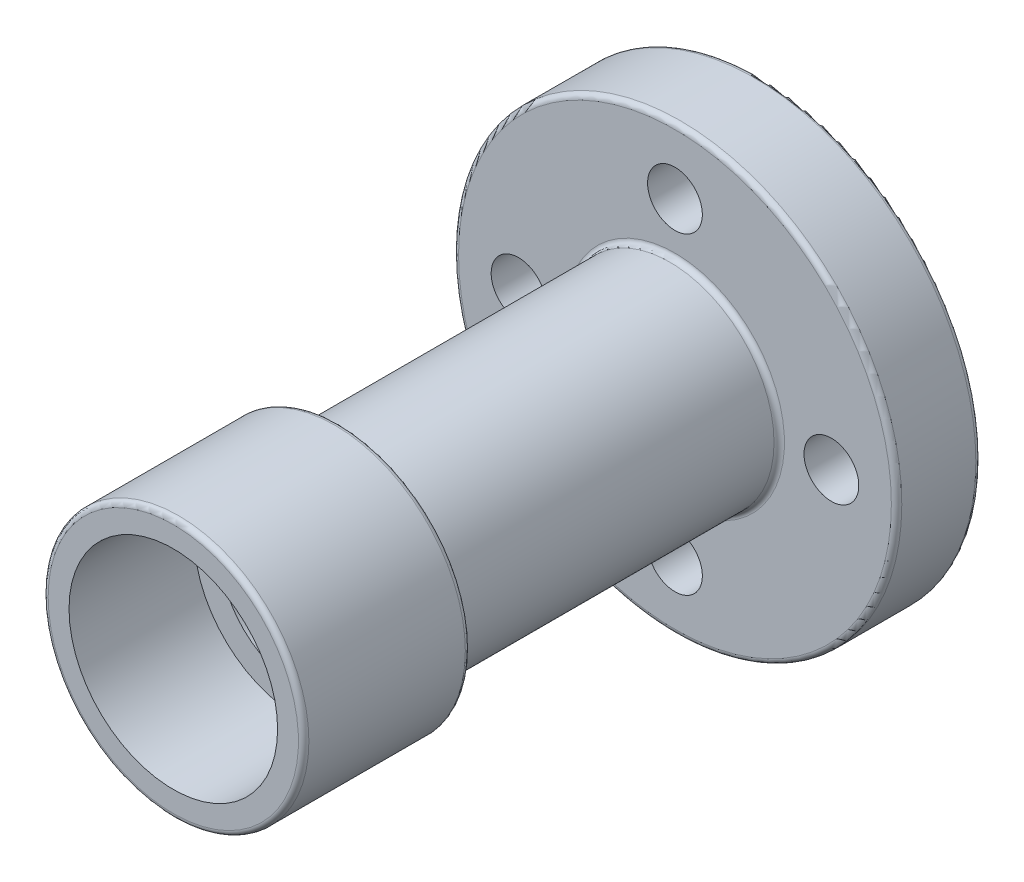
ISO-10303-21;
HEADER;
FILE_DESCRIPTION(('STEP AP214'),'2;1');
FILE_NAME('part.step','',(''),(''),'','','');
FILE_SCHEMA(('AUTOMOTIVE_DESIGN { 1 0 10303 214 1 1 1 1 }'));
ENDSEC;
DATA;
#1=APPLICATION_CONTEXT('core data for automotive mechanical design processes');
#2=APPLICATION_PROTOCOL_DEFINITION('international standard','automotive_design',2000,#1);
#3=PRODUCT_CONTEXT('',#1,'mechanical');
#4=PRODUCT('Part','Part','',(#3));
#5=PRODUCT_RELATED_PRODUCT_CATEGORY('part','',(#4));
#6=PRODUCT_DEFINITION_FORMATION('','',#4);
#7=PRODUCT_DEFINITION_CONTEXT('part definition',#1,'design');
#8=PRODUCT_DEFINITION('design','',#6,#7);
#9=PRODUCT_DEFINITION_SHAPE('','',#8);
#10=(LENGTH_UNIT() NAMED_UNIT(*) SI_UNIT(.MILLI.,.METRE.));
#11=(NAMED_UNIT(*) PLANE_ANGLE_UNIT() SI_UNIT($,.RADIAN.));
#12=(NAMED_UNIT(*) SI_UNIT($,.STERADIAN.) SOLID_ANGLE_UNIT());
#13=UNCERTAINTY_MEASURE_WITH_UNIT(LENGTH_MEASURE(1.E-05),#10,'distance_accuracy_value','');
#14=(GEOMETRIC_REPRESENTATION_CONTEXT(3) GLOBAL_UNCERTAINTY_ASSIGNED_CONTEXT((#13)) GLOBAL_UNIT_ASSIGNED_CONTEXT((#10,
#11,#12)) REPRESENTATION_CONTEXT('',''));
#15=CARTESIAN_POINT('',(0.,0.,0.));
#16=DIRECTION('',(0.,0.,1.));
#17=DIRECTION('',(1.,0.,0.));
#18=AXIS2_PLACEMENT_3D('',#15,#16,#17);
#19=CARTESIAN_POINT('',(0.,0.,511.464555615893));
#20=DIRECTION('',(0.,0.,1.));
#21=DIRECTION('',(1.,0.,0.));
#22=AXIS2_PLACEMENT_3D('',#19,#20,#21);
#23=CYLINDRICAL_SURFACE('',#22,15.);
#24=CARTESIAN_POINT('',(0.,0.,3.));
#25=DIRECTION('',(0.,0.,1.));
#26=DIRECTION('',(1.,0.,0.));
#27=AXIS2_PLACEMENT_3D('',#24,#25,#26);
#28=CIRCLE('',#27,15.);
#29=CARTESIAN_POINT('',(15.,0.,3.));
#30=VERTEX_POINT('',#29);
#31=EDGE_CURVE('E84',#30,#30,#28,.F.);
#32=ORIENTED_EDGE('',*,*,#31,.T.);
#33=EDGE_LOOP('',(#32));
#34=FACE_BOUND('',#33,.T.);
#35=CARTESIAN_POINT('',(0.,0.,88.4));
#36=DIRECTION('',(0.,0.,1.));
#37=DIRECTION('',(1.,0.,0.));
#38=AXIS2_PLACEMENT_3D('',#35,#36,#37);
#39=CIRCLE('',#38,15.);
#40=CARTESIAN_POINT('',(15.,0.,88.4));
#41=VERTEX_POINT('',#40);
#42=EDGE_CURVE('E91',#41,#41,#39,.T.);
#43=ORIENTED_EDGE('',*,*,#42,.T.);
#44=EDGE_LOOP('',(#43));
#45=FACE_BOUND('',#44,.T.);
#46=ADVANCED_FACE('F39',(#34,#45),#23,.F.);
#47=CARTESIAN_POINT('',(0.,15.,0.));
#48=DIRECTION('',(0.,0.,1.));
#49=DIRECTION('',(1.,0.,0.));
#50=AXIS2_PLACEMENT_3D('',#47,#48,#49);
#51=PLANE('',#50);
#52=CARTESIAN_POINT('',(0.,0.,0.));
#53=DIRECTION('',(0.,0.,1.));
#54=DIRECTION('',(1.,0.,0.));
#55=AXIS2_PLACEMENT_3D('',#52,#53,#54);
#56=CIRCLE('',#55,41.5);
#57=CARTESIAN_POINT('',(41.5,0.,0.));
#58=VERTEX_POINT('',#57);
#59=EDGE_CURVE('E10',#58,#58,#56,.F.);
#60=ORIENTED_EDGE('',*,*,#59,.T.);
#61=EDGE_LOOP('',(#60));
#62=FACE_BOUND('',#61,.T.);
#63=CARTESIAN_POINT('',(0.,0.,0.));
#64=DIRECTION('',(0.,0.,1.));
#65=DIRECTION('',(1.,0.,0.));
#66=AXIS2_PLACEMENT_3D('',#63,#64,#65);
#67=CIRCLE('',#66,18.);
#68=CARTESIAN_POINT('',(18.,0.,0.));
#69=VERTEX_POINT('',#68);
#70=EDGE_CURVE('E88',#69,#69,#67,.T.);
#71=ORIENTED_EDGE('',*,*,#70,.T.);
#72=EDGE_LOOP('',(#71));
#73=FACE_BOUND('',#72,.T.);
#74=CARTESIAN_POINT('',(0.,30.,0.));
#75=DIRECTION('',(0.,0.,-1.));
#76=DIRECTION('',(-1.,0.,0.));
#77=AXIS2_PLACEMENT_3D('',#74,#75,#76);
#78=CIRCLE('',#77,5.25);
#79=CARTESIAN_POINT('',(-5.25,30.,0.));
#80=VERTEX_POINT('',#79);
#81=EDGE_CURVE('E103',#80,#80,#78,.T.);
#82=ORIENTED_EDGE('',*,*,#81,.F.);
#83=EDGE_LOOP('',(#82));
#84=FACE_BOUND('',#83,.T.);
#85=CARTESIAN_POINT('',(-30.,0.,0.));
#86=DIRECTION('',(0.,0.,-1.));
#87=DIRECTION('',(-1.,0.,0.));
#88=AXIS2_PLACEMENT_3D('',#85,#86,#87);
#89=CIRCLE('',#88,5.25);
#90=CARTESIAN_POINT('',(-35.25,0.,0.));
#91=VERTEX_POINT('',#90);
#92=EDGE_CURVE('E117',#91,#91,#89,.T.);
#93=ORIENTED_EDGE('',*,*,#92,.F.);
#94=EDGE_LOOP('',(#93));
#95=FACE_BOUND('',#94,.T.);
#96=CARTESIAN_POINT('',(0.,-30.,0.));
#97=DIRECTION('',(0.,0.,-1.));
#98=DIRECTION('',(-1.,0.,0.));
#99=AXIS2_PLACEMENT_3D('',#96,#97,#98);
#100=CIRCLE('',#99,5.25);
#101=CARTESIAN_POINT('',(-5.25,-30.,0.));
#102=VERTEX_POINT('',#101);
#103=EDGE_CURVE('E111',#102,#102,#100,.T.);
#104=ORIENTED_EDGE('',*,*,#103,.F.);
#105=EDGE_LOOP('',(#104));
#106=FACE_BOUND('',#105,.T.);
#107=CARTESIAN_POINT('',(30.,0.,0.));
#108=DIRECTION('',(0.,0.,-1.));
#109=DIRECTION('',(-1.,0.,0.));
#110=AXIS2_PLACEMENT_3D('',#107,#108,#109);
#111=CIRCLE('',#110,5.24999999999912);
#112=CARTESIAN_POINT('',(24.7500000000009,0.,0.));
#113=VERTEX_POINT('',#112);
#114=EDGE_CURVE('E112',#113,#113,#111,.T.);
#115=ORIENTED_EDGE('',*,*,#114,.F.);
#116=EDGE_LOOP('',(#115));
#117=FACE_BOUND('',#116,.T.);
#118=ADVANCED_FACE('F127',(#62,#73,#84,#95,#106,#117),#51,.F.);
#119=CARTESIAN_POINT('',(0.,0.,511.464555615893));
#120=DIRECTION('',(0.,0.,1.));
#121=DIRECTION('',(1.,0.,0.));
#122=AXIS2_PLACEMENT_3D('',#119,#120,#121);
#123=CYLINDRICAL_SURFACE('',#122,42.5);
#124=CARTESIAN_POINT('',(0.,0.,15.2));
#125=DIRECTION('',(0.,0.,-1.));
#126=DIRECTION('',(-1.,0.,0.));
#127=AXIS2_PLACEMENT_3D('',#124,#125,#126);
#128=CIRCLE('',#127,42.5);
#129=CARTESIAN_POINT('',(-42.5,0.,15.2));
#130=VERTEX_POINT('',#129);
#131=EDGE_CURVE('E46',#130,#130,#128,.T.);
#132=ORIENTED_EDGE('',*,*,#131,.T.);
#133=EDGE_LOOP('',(#132));
#134=FACE_BOUND('',#133,.T.);
#135=CARTESIAN_POINT('',(0.,0.,1.));
#136=DIRECTION('',(0.,0.,1.));
#137=DIRECTION('',(1.,0.,0.));
#138=AXIS2_PLACEMENT_3D('',#135,#136,#137);
#139=CIRCLE('',#138,42.5);
#140=CARTESIAN_POINT('',(42.5,0.,1.));
#141=VERTEX_POINT('',#140);
#142=EDGE_CURVE('E49',#141,#141,#139,.T.);
#143=ORIENTED_EDGE('',*,*,#142,.T.);
#144=EDGE_LOOP('',(#143));
#145=FACE_BOUND('',#144,.T.);
#146=ADVANCED_FACE('F129',(#134,#145),#123,.T.);
#147=CARTESIAN_POINT('',(0.,42.5,16.2));
#148=DIRECTION('',(0.,0.,-1.));
#149=DIRECTION('',(-1.,0.,0.));
#150=AXIS2_PLACEMENT_3D('',#147,#148,#149);
#151=PLANE('',#150);
#152=CARTESIAN_POINT('',(0.,0.,16.2));
#153=DIRECTION('',(0.,0.,-1.));
#154=DIRECTION('',(-1.,0.,0.));
#155=AXIS2_PLACEMENT_3D('',#152,#153,#154);
#156=CIRCLE('',#155,21.);
#157=CARTESIAN_POINT('',(-21.,0.,16.2));
#158=VERTEX_POINT('',#157);
#159=EDGE_CURVE('E53',#158,#158,#156,.T.);
#160=ORIENTED_EDGE('',*,*,#159,.T.);
#161=EDGE_LOOP('',(#160));
#162=FACE_BOUND('',#161,.T.);
#163=CARTESIAN_POINT('',(0.,0.,16.2));
#164=DIRECTION('',(0.,0.,-1.));
#165=DIRECTION('',(-1.,0.,0.));
#166=AXIS2_PLACEMENT_3D('',#163,#164,#165);
#167=CIRCLE('',#166,41.5);
#168=CARTESIAN_POINT('',(-41.5,0.,16.2));
#169=VERTEX_POINT('',#168);
#170=EDGE_CURVE('E56',#169,#169,#167,.F.);
#171=ORIENTED_EDGE('',*,*,#170,.T.);
#172=EDGE_LOOP('',(#171));
#173=FACE_BOUND('',#172,.T.);
#174=CARTESIAN_POINT('',(0.,30.,16.2));
#175=DIRECTION('',(0.,0.,-1.));
#176=DIRECTION('',(-1.,0.,0.));
#177=AXIS2_PLACEMENT_3D('',#174,#175,#176);
#178=CIRCLE('',#177,5.25);
#179=CARTESIAN_POINT('',(-5.25,30.,16.2));
#180=VERTEX_POINT('',#179);
#181=EDGE_CURVE('E89',#180,#180,#178,.T.);
#182=ORIENTED_EDGE('',*,*,#181,.T.);
#183=EDGE_LOOP('',(#182));
#184=FACE_BOUND('',#183,.T.);
#185=CARTESIAN_POINT('',(-30.,0.,16.2));
#186=DIRECTION('',(0.,0.,-1.));
#187=DIRECTION('',(-1.,0.,0.));
#188=AXIS2_PLACEMENT_3D('',#185,#186,#187);
#189=CIRCLE('',#188,5.25);
#190=CARTESIAN_POINT('',(-35.25,0.,16.2));
#191=VERTEX_POINT('',#190);
#192=EDGE_CURVE('E94',#191,#191,#189,.T.);
#193=ORIENTED_EDGE('',*,*,#192,.T.);
#194=EDGE_LOOP('',(#193));
#195=FACE_BOUND('',#194,.T.);
#196=CARTESIAN_POINT('',(0.,-30.,16.2));
#197=DIRECTION('',(0.,0.,-1.));
#198=DIRECTION('',(-1.,0.,0.));
#199=AXIS2_PLACEMENT_3D('',#196,#197,#198);
#200=CIRCLE('',#199,5.25);
#201=CARTESIAN_POINT('',(-5.25,-30.,16.2));
#202=VERTEX_POINT('',#201);
#203=EDGE_CURVE('E100',#202,#202,#200,.T.);
#204=ORIENTED_EDGE('',*,*,#203,.T.);
#205=EDGE_LOOP('',(#204));
#206=FACE_BOUND('',#205,.T.);
#207=CARTESIAN_POINT('',(30.,0.,16.2));
#208=DIRECTION('',(0.,0.,-1.));
#209=DIRECTION('',(-1.,0.,0.));
#210=AXIS2_PLACEMENT_3D('',#207,#208,#209);
#211=CIRCLE('',#210,5.24999999999912);
#212=CARTESIAN_POINT('',(24.7500000000009,0.,16.2));
#213=VERTEX_POINT('',#212);
#214=EDGE_CURVE('E99',#213,#213,#211,.T.);
#215=ORIENTED_EDGE('',*,*,#214,.T.);
#216=EDGE_LOOP('',(#215));
#217=FACE_BOUND('',#216,.T.);
#218=ADVANCED_FACE('F144',(#162,#173,#184,#195,#206,#217),#151,.F.);
#219=CARTESIAN_POINT('',(0.,0.,511.464555615893));
#220=DIRECTION('',(0.,0.,1.));
#221=DIRECTION('',(1.,0.,0.));
#222=AXIS2_PLACEMENT_3D('',#219,#220,#221);
#223=CYLINDRICAL_SURFACE('',#222,20.);
#224=CARTESIAN_POINT('',(0.,0.,79.4));
#225=DIRECTION('',(0.,0.,1.));
#226=DIRECTION('',(1.,0.,0.));
#227=AXIS2_PLACEMENT_3D('',#224,#225,#226);
#228=CIRCLE('',#227,20.);
#229=CARTESIAN_POINT('',(20.,0.,79.4));
#230=VERTEX_POINT('',#229);
#231=EDGE_CURVE('E72',#230,#230,#228,.F.);
#232=ORIENTED_EDGE('',*,*,#231,.T.);
#233=EDGE_LOOP('',(#232));
#234=FACE_BOUND('',#233,.T.);
#235=CARTESIAN_POINT('',(0.,0.,17.2));
#236=DIRECTION('',(0.,0.,-1.));
#237=DIRECTION('',(-1.,0.,0.));
#238=AXIS2_PLACEMENT_3D('',#235,#236,#237);
#239=CIRCLE('',#238,20.);
#240=CARTESIAN_POINT('',(-20.,0.,17.2));
#241=VERTEX_POINT('',#240);
#242=EDGE_CURVE('E74',#241,#241,#239,.F.);
#243=ORIENTED_EDGE('',*,*,#242,.T.);
#244=EDGE_LOOP('',(#243));
#245=FACE_BOUND('',#244,.T.);
#246=ADVANCED_FACE('F150',(#234,#245),#223,.T.);
#247=CARTESIAN_POINT('',(0.,20.,80.4));
#248=DIRECTION('',(0.,0.,1.));
#249=DIRECTION('',(1.,0.,0.));
#250=AXIS2_PLACEMENT_3D('',#247,#248,#249);
#251=PLANE('',#250);
#252=CARTESIAN_POINT('',(0.,0.,80.4));
#253=DIRECTION('',(0.,0.,1.));
#254=DIRECTION('',(1.,0.,0.));
#255=AXIS2_PLACEMENT_3D('',#252,#253,#254);
#256=CIRCLE('',#255,21.);
#257=CARTESIAN_POINT('',(21.,0.,80.4));
#258=VERTEX_POINT('',#257);
#259=EDGE_CURVE('E77',#258,#258,#256,.T.);
#260=ORIENTED_EDGE('',*,*,#259,.T.);
#261=EDGE_LOOP('',(#260));
#262=FACE_BOUND('',#261,.T.);
#263=CARTESIAN_POINT('',(0.,0.,80.4));
#264=DIRECTION('',(0.,0.,1.));
#265=DIRECTION('',(1.,0.,0.));
#266=AXIS2_PLACEMENT_3D('',#263,#264,#265);
#267=CIRCLE('',#266,24.);
#268=CARTESIAN_POINT('',(24.,0.,80.4));
#269=VERTEX_POINT('',#268);
#270=EDGE_CURVE('E80',#269,#269,#267,.F.);
#271=ORIENTED_EDGE('',*,*,#270,.T.);
#272=EDGE_LOOP('',(#271));
#273=FACE_BOUND('',#272,.T.);
#274=ADVANCED_FACE('F152',(#262,#273),#251,.F.);
#275=CARTESIAN_POINT('',(0.,0.,511.464555615893));
#276=DIRECTION('',(0.,0.,1.));
#277=DIRECTION('',(1.,0.,0.));
#278=AXIS2_PLACEMENT_3D('',#275,#276,#277);
#279=CYLINDRICAL_SURFACE('',#278,25.);
#280=CARTESIAN_POINT('',(0.,0.,111.4));
#281=DIRECTION('',(0.,0.,-1.));
#282=DIRECTION('',(-1.,0.,0.));
#283=AXIS2_PLACEMENT_3D('',#280,#281,#282);
#284=CIRCLE('',#283,25.);
#285=CARTESIAN_POINT('',(-25.,0.,111.4));
#286=VERTEX_POINT('',#285);
#287=EDGE_CURVE('E62',#286,#286,#284,.T.);
#288=ORIENTED_EDGE('',*,*,#287,.T.);
#289=EDGE_LOOP('',(#288));
#290=FACE_BOUND('',#289,.T.);
#291=CARTESIAN_POINT('',(0.,0.,81.4));
#292=DIRECTION('',(0.,0.,1.));
#293=DIRECTION('',(1.,0.,0.));
#294=AXIS2_PLACEMENT_3D('',#291,#292,#293);
#295=CIRCLE('',#294,25.);
#296=CARTESIAN_POINT('',(25.,0.,81.4));
#297=VERTEX_POINT('',#296);
#298=EDGE_CURVE('E65',#297,#297,#295,.T.);
#299=ORIENTED_EDGE('',*,*,#298,.T.);
#300=EDGE_LOOP('',(#299));
#301=FACE_BOUND('',#300,.T.);
#302=ADVANCED_FACE('F226',(#290,#301),#279,.T.);
#303=CARTESIAN_POINT('',(0.,25.,112.4));
#304=DIRECTION('',(0.,0.,-1.));
#305=DIRECTION('',(-1.,0.,0.));
#306=AXIS2_PLACEMENT_3D('',#303,#304,#305);
#307=PLANE('',#306);
#308=CARTESIAN_POINT('',(0.,0.,112.4));
#309=DIRECTION('',(0.,0.,-1.));
#310=DIRECTION('',(-1.,0.,0.));
#311=AXIS2_PLACEMENT_3D('',#308,#309,#310);
#312=CIRCLE('',#311,24.);
#313=CARTESIAN_POINT('',(-24.,0.,112.4));
#314=VERTEX_POINT('',#313);
#315=EDGE_CURVE('E69',#314,#314,#312,.F.);
#316=ORIENTED_EDGE('',*,*,#315,.T.);
#317=EDGE_LOOP('',(#316));
#318=FACE_BOUND('',#317,.T.);
#319=CARTESIAN_POINT('',(0.,0.,112.4));
#320=DIRECTION('',(0.,0.,1.));
#321=DIRECTION('',(1.,0.,0.));
#322=AXIS2_PLACEMENT_3D('',#319,#320,#321);
#323=CIRCLE('',#322,20.);
#324=CARTESIAN_POINT('',(20.,0.,112.4));
#325=VERTEX_POINT('',#324);
#326=EDGE_CURVE('E90',#325,#325,#323,.T.);
#327=ORIENTED_EDGE('',*,*,#326,.F.);
#328=EDGE_LOOP('',(#327));
#329=FACE_BOUND('',#328,.T.);
#330=ADVANCED_FACE('F225',(#318,#329),#307,.F.);
#331=CARTESIAN_POINT('',(0.,0.,511.464555615893));
#332=DIRECTION('',(0.,0.,1.));
#333=DIRECTION('',(1.,0.,0.));
#334=AXIS2_PLACEMENT_3D('',#331,#332,#333);
#335=CYLINDRICAL_SURFACE('',#334,20.);
#336=CARTESIAN_POINT('',(0.,0.,88.4));
#337=DIRECTION('',(0.,0.,1.));
#338=DIRECTION('',(1.,0.,0.));
#339=AXIS2_PLACEMENT_3D('',#336,#337,#338);
#340=CIRCLE('',#339,20.);
#341=CARTESIAN_POINT('',(20.,0.,88.4));
#342=VERTEX_POINT('',#341);
#343=EDGE_CURVE('E106',#342,#342,#340,.T.);
#344=ORIENTED_EDGE('',*,*,#343,.F.);
#345=EDGE_LOOP('',(#344));
#346=FACE_BOUND('',#345,.T.);
#347=ORIENTED_EDGE('',*,*,#326,.T.);
#348=EDGE_LOOP('',(#347));
#349=FACE_BOUND('',#348,.T.);
#350=ADVANCED_FACE('F217',(#346,#349),#335,.F.);
#351=CARTESIAN_POINT('',(0.,20.,88.4));
#352=DIRECTION('',(0.,0.,-1.));
#353=DIRECTION('',(-1.,0.,0.));
#354=AXIS2_PLACEMENT_3D('',#351,#352,#353);
#355=PLANE('',#354);
#356=ORIENTED_EDGE('',*,*,#42,.F.);
#357=EDGE_LOOP('',(#356));
#358=FACE_BOUND('',#357,.T.);
#359=ORIENTED_EDGE('',*,*,#343,.T.);
#360=EDGE_LOOP('',(#359));
#361=FACE_BOUND('',#360,.T.);
#362=ADVANCED_FACE('F143',(#358,#361),#355,.F.);
#363=CARTESIAN_POINT('',(30.,0.,39.));
#364=DIRECTION('',(0.,0.,-1.));
#365=DIRECTION('',(-1.,0.,0.));
#366=AXIS2_PLACEMENT_3D('',#363,#364,#365);
#367=CYLINDRICAL_SURFACE('',#366,5.24999999999912);
#368=ORIENTED_EDGE('',*,*,#114,.T.);
#369=EDGE_LOOP('',(#368));
#370=FACE_BOUND('',#369,.T.);
#371=ORIENTED_EDGE('',*,*,#214,.F.);
#372=EDGE_LOOP('',(#371));
#373=FACE_BOUND('',#372,.T.);
#374=ADVANCED_FACE('F137',(#370,#373),#367,.F.);
#375=CARTESIAN_POINT('',(0.,-30.,39.));
#376=DIRECTION('',(0.,0.,-1.));
#377=DIRECTION('',(-1.,0.,0.));
#378=AXIS2_PLACEMENT_3D('',#375,#376,#377);
#379=CYLINDRICAL_SURFACE('',#378,5.25);
#380=ORIENTED_EDGE('',*,*,#103,.T.);
#381=EDGE_LOOP('',(#380));
#382=FACE_BOUND('',#381,.T.);
#383=ORIENTED_EDGE('',*,*,#203,.F.);
#384=EDGE_LOOP('',(#383));
#385=FACE_BOUND('',#384,.T.);
#386=ADVANCED_FACE('F140',(#382,#385),#379,.F.);
#387=CARTESIAN_POINT('',(-30.,0.,39.));
#388=DIRECTION('',(0.,0.,-1.));
#389=DIRECTION('',(-1.,0.,0.));
#390=AXIS2_PLACEMENT_3D('',#387,#388,#389);
#391=CYLINDRICAL_SURFACE('',#390,5.25);
#392=ORIENTED_EDGE('',*,*,#92,.T.);
#393=EDGE_LOOP('',(#392));
#394=FACE_BOUND('',#393,.T.);
#395=ORIENTED_EDGE('',*,*,#192,.F.);
#396=EDGE_LOOP('',(#395));
#397=FACE_BOUND('',#396,.T.);
#398=ADVANCED_FACE('F206',(#394,#397),#391,.F.);
#399=CARTESIAN_POINT('',(0.,30.,39.));
#400=DIRECTION('',(0.,0.,-1.));
#401=DIRECTION('',(-1.,0.,0.));
#402=AXIS2_PLACEMENT_3D('',#399,#400,#401);
#403=CYLINDRICAL_SURFACE('',#402,5.25);
#404=ORIENTED_EDGE('',*,*,#81,.T.);
#405=EDGE_LOOP('',(#404));
#406=FACE_BOUND('',#405,.T.);
#407=ORIENTED_EDGE('',*,*,#181,.F.);
#408=EDGE_LOOP('',(#407));
#409=FACE_BOUND('',#408,.T.);
#410=ADVANCED_FACE('F124',(#406,#409),#403,.F.);
#411=CARTESIAN_POINT('',(0.,0.,0.));
#412=DIRECTION('',(0.,0.,-1.));
#413=DIRECTION('',(-1.,0.,0.));
#414=AXIS2_PLACEMENT_3D('',#411,#412,#413);
#415=CONICAL_SURFACE('',#414,18.,0.785398163397448);
#416=ORIENTED_EDGE('',*,*,#31,.F.);
#417=EDGE_LOOP('',(#416));
#418=FACE_BOUND('',#417,.T.);
#419=ORIENTED_EDGE('',*,*,#70,.F.);
#420=EDGE_LOOP('',(#419));
#421=FACE_BOUND('',#420,.T.);
#422=ADVANCED_FACE('F166',(#418,#421),#415,.F.);
#423=CARTESIAN_POINT('',(0.,0.,79.4));
#424=DIRECTION('',(0.,0.,1.));
#425=DIRECTION('',(1.,0.,0.));
#426=AXIS2_PLACEMENT_3D('',#423,#424,#425);
#427=TOROIDAL_SURFACE('',#426,21.,1.);
#428=ORIENTED_EDGE('',*,*,#231,.F.);
#429=EDGE_LOOP('',(#428));
#430=FACE_BOUND('',#429,.T.);
#431=ORIENTED_EDGE('',*,*,#259,.F.);
#432=EDGE_LOOP('',(#431));
#433=FACE_BOUND('',#432,.T.);
#434=ADVANCED_FACE('F174',(#430,#433),#427,.F.);
#435=CARTESIAN_POINT('',(0.,0.,111.4));
#436=DIRECTION('',(0.,0.,-1.));
#437=DIRECTION('',(-1.,0.,0.));
#438=AXIS2_PLACEMENT_3D('',#435,#436,#437);
#439=TOROIDAL_SURFACE('',#438,24.,1.);
#440=ORIENTED_EDGE('',*,*,#287,.F.);
#441=EDGE_LOOP('',(#440));
#442=FACE_BOUND('',#441,.T.);
#443=ORIENTED_EDGE('',*,*,#315,.F.);
#444=EDGE_LOOP('',(#443));
#445=FACE_BOUND('',#444,.T.);
#446=ADVANCED_FACE('F177',(#442,#445),#439,.T.);
#447=CARTESIAN_POINT('',(0.,0.,81.4));
#448=DIRECTION('',(0.,0.,1.));
#449=DIRECTION('',(1.,0.,0.));
#450=AXIS2_PLACEMENT_3D('',#447,#448,#449);
#451=TOROIDAL_SURFACE('',#450,24.,1.);
#452=ORIENTED_EDGE('',*,*,#270,.F.);
#453=EDGE_LOOP('',(#452));
#454=FACE_BOUND('',#453,.T.);
#455=ORIENTED_EDGE('',*,*,#298,.F.);
#456=EDGE_LOOP('',(#455));
#457=FACE_BOUND('',#456,.T.);
#458=ADVANCED_FACE('F182',(#454,#457),#451,.T.);
#459=CARTESIAN_POINT('',(0.,0.,17.2));
#460=DIRECTION('',(0.,0.,-1.));
#461=DIRECTION('',(-1.,0.,0.));
#462=AXIS2_PLACEMENT_3D('',#459,#460,#461);
#463=TOROIDAL_SURFACE('',#462,21.,1.);
#464=ORIENTED_EDGE('',*,*,#159,.F.);
#465=EDGE_LOOP('',(#464));
#466=FACE_BOUND('',#465,.T.);
#467=ORIENTED_EDGE('',*,*,#242,.F.);
#468=EDGE_LOOP('',(#467));
#469=FACE_BOUND('',#468,.T.);
#470=ADVANCED_FACE('F183',(#466,#469),#463,.F.);
#471=CARTESIAN_POINT('',(0.,0.,15.2));
#472=DIRECTION('',(0.,0.,-1.));
#473=DIRECTION('',(-1.,0.,0.));
#474=AXIS2_PLACEMENT_3D('',#471,#472,#473);
#475=TOROIDAL_SURFACE('',#474,41.5,1.);
#476=ORIENTED_EDGE('',*,*,#131,.F.);
#477=EDGE_LOOP('',(#476));
#478=FACE_BOUND('',#477,.T.);
#479=ORIENTED_EDGE('',*,*,#170,.F.);
#480=EDGE_LOOP('',(#479));
#481=FACE_BOUND('',#480,.T.);
#482=ADVANCED_FACE('F189',(#478,#481),#475,.T.);
#483=CARTESIAN_POINT('',(0.,0.,1.));
#484=DIRECTION('',(0.,0.,1.));
#485=DIRECTION('',(1.,0.,0.));
#486=AXIS2_PLACEMENT_3D('',#483,#484,#485);
#487=TOROIDAL_SURFACE('',#486,41.5,1.);
#488=ORIENTED_EDGE('',*,*,#59,.F.);
#489=EDGE_LOOP('',(#488));
#490=FACE_BOUND('',#489,.T.);
#491=ORIENTED_EDGE('',*,*,#142,.F.);
#492=EDGE_LOOP('',(#491));
#493=FACE_BOUND('',#492,.T.);
#494=ADVANCED_FACE('F41',(#490,#493),#487,.T.);
#495=CLOSED_SHELL('',(#46,#118,#146,#218,#246,#274,#302,#330,#350,#362,#374,#386,#398,#410,#422,
#434,#446,#458,#470,#482,#494));
#496=MANIFOLD_SOLID_BREP('B2',#495);
#497=ADVANCED_BREP_SHAPE_REPRESENTATION('',(#18,#496),#14);
#498=SHAPE_DEFINITION_REPRESENTATION(#9,#497);
ENDSEC;
END-ISO-10303-21;
